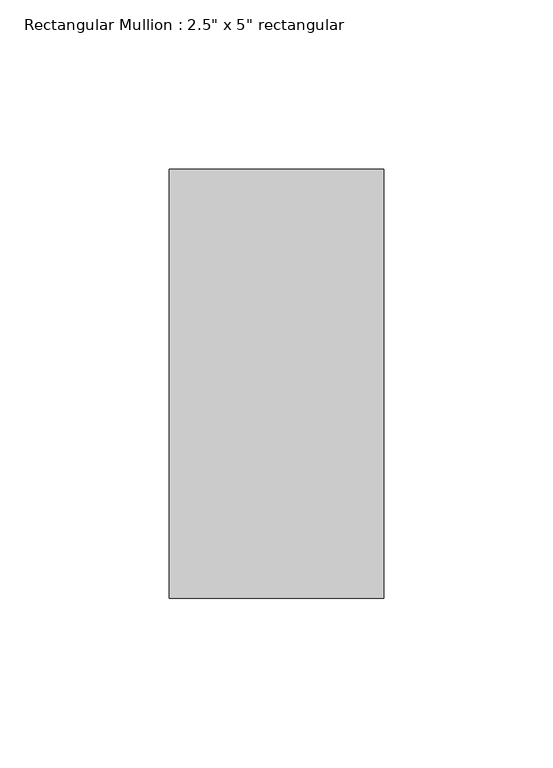
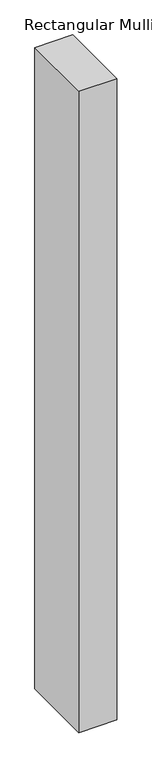
"""IFC4 building model written with IfcOpenShell, lengths in millimetres: member geometry."""

from ifc_helpers import new_model, si_unit, frame, origin, place, context, project, spatial, polyline, outline, extrude, source, transform, mapped, element, save


def member_43f490c4(model_context):
    return source(origin(), model_context, "Body", "SweptSolid", [
        extrude(outline(polyline([(0.0, 63.5), (0.0, -63.5), (-63.5, -63.5), (-63.5, 63.5), (0.0, 63.5)])), frame((0.0, 0.0, -1132.4166667), z_axis=(0.0, 0.0, 1.0), x_axis=(1.0, 0.0, 0.0)), (0.0, 0.0, 1.0), 1132.4166667),
    ])


if __name__ == "__main__":
    model = new_model("IFC4")
    model_context = context("Model", 3, world=origin())
    ifc_project = project(units=[si_unit("LENGTHUNIT", "METRE", prefix="MILLI")], contexts=[model_context])
    site = spatial("IfcSite", under=ifc_project)
    building = spatial("IfcBuilding", under=site)
    placement = place(None, origin())
    member_shape = member_43f490c4(model_context)
    element("IfcMember", 1, ObjectType="Rectangular Mullion : 2.5\" x 5\" rectangular", at=placement, inside=building, context=model_context, shape_type="MappedRepresentation", body=[
        mapped(member_shape, transform((0.0, 0.0, 0.0), x_axis=(1.0, 0.0, 0.0), y_axis=(0.0, 1.0, 0.0), z_axis=(0.0, 0.0, 1.0))),
    ])
    save(model, "model.ifc")

# Revit data of these elements
# Type "Rectangular Mullion : 2.5\" x 5\" rectangular"
#   built-in parameter 1007304 = 0.416667 (stored number, unit not read)
#   built-in parameter 1007301 = 0.104167 (stored number, unit not read)
#   built-in parameter 1007300 = 0.104167 (stored number, unit not read)
# Element 1 (IfcMember, "Rectangular Mullion : 2.5\" x 5\" rectangular")
#   Materials on its faces: "Aluminum"
# Materials
#   "Aluminum": class "Metal", colour RGB 247 247 247, transparency 0, Description = "Aluminum 6061", Cost = 0
